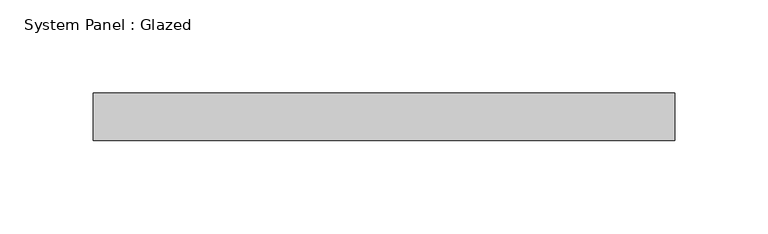
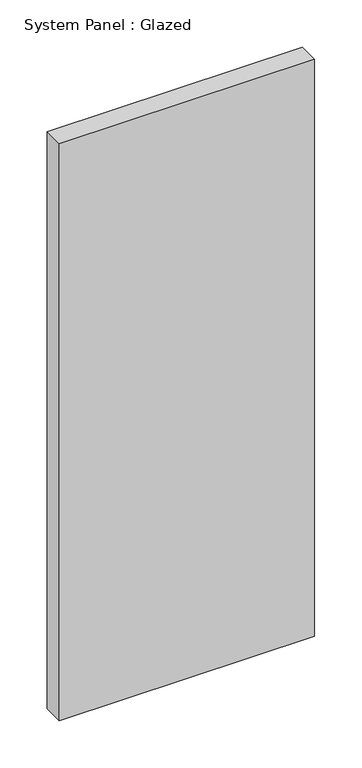
"""IFC4 building model written with IfcOpenShell, lengths in millimetres: plate geometry, System Panel : Glazed."""

from ifc_helpers import new_model, si_unit, origin, origin_with_axes, place, context, project, spatial, polyline, outline, extrude, source, transform, mapped, element, save


def system_panel_glazed_51dabc0a(model_context):
    return source(origin(), model_context, "Body", "SweptSolid", [
        extrude(outline(polyline([(155.575, 19.05), (-155.575, 19.05), (-155.575, 44.45), (155.575, 44.45), (155.575, 19.05)])), origin_with_axes(), (0.0, 0.0, 1.0), 742.95),
    ])


if __name__ == "__main__":
    model = new_model("IFC4")
    model_context = context("Model", 3, world=origin())
    ifc_project = project(units=[si_unit("LENGTHUNIT", "METRE", prefix="MILLI")], contexts=[model_context])
    site = spatial("IfcSite", under=ifc_project)
    building = spatial("IfcBuilding", under=site)
    placement = place(None, origin())
    system_panel_glazed_shape = system_panel_glazed_51dabc0a(model_context)
    element("IfcPlate", 1, ObjectType="System Panel : Glazed", at=placement, inside=building, context=model_context, shape_type="MappedRepresentation", body=[
        mapped(system_panel_glazed_shape, transform((0.0, 0.0, 0.0), x_axis=(1.0, 0.0, 0.0), y_axis=(0.0, 1.0, 0.0), z_axis=(0.0, 0.0, 1.0))),
    ])
    save(model, "model.ifc")

# Revit data of these elements
# Type "System Panel : Glazed"
#   Construction Type Id = "GSP4R"
#   Analytic Construction = "1/8 in Pilkington single glazing"
#   Visual Light Transmittance = 0.9
#   Solar Heat Gain Coefficient = 0.86
#   Heat Transfer Coefficient (U) = 1.18115 BTU/(h·ft²·°F)
# Element 1 (IfcPlate, "System Panel : Glazed")
#   Materials on its faces: "Glass"
# Materials
#   "Glass": class "Glass", colour RGB 0 128 192, transparency 0.75, Description = "Soda Lime Glass", Cost = 0
